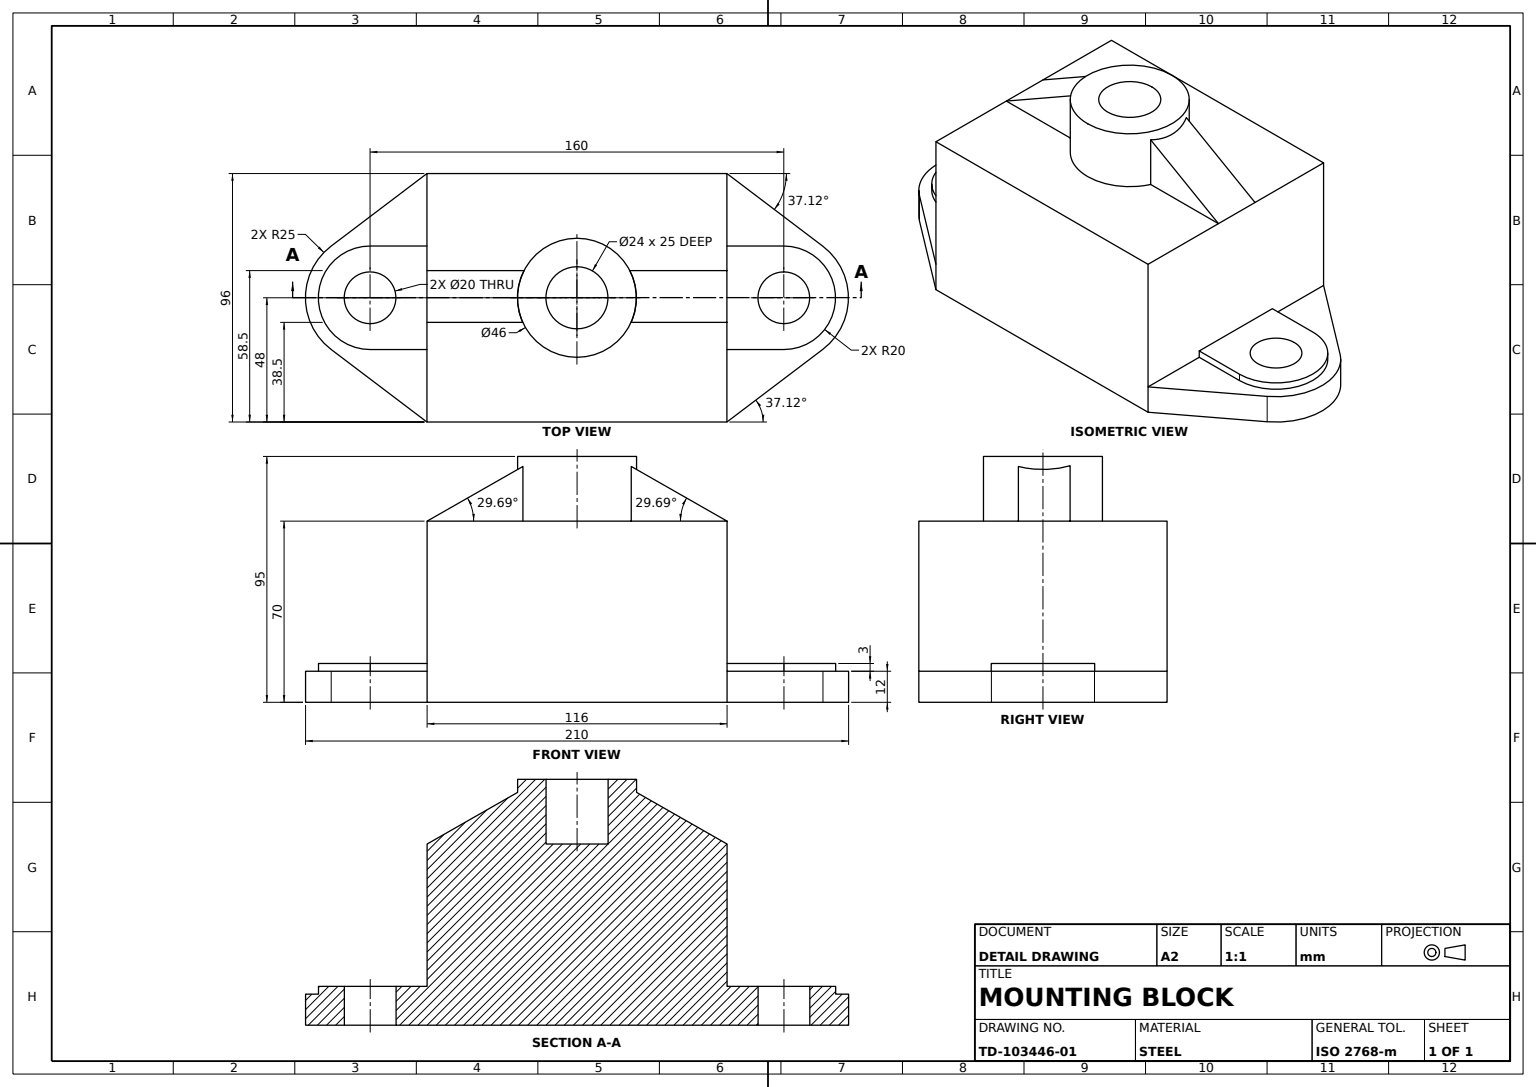
from build123d import *

# Parameters (mm, degrees)
HOUSING_BLOCK_SKETCH_W = 116
HOUSING_BLOCK_SKETCH_H = 70
HOUSING_BLOCK_DEPTH    = 96
MOUNTING_FLANGE_DEPTH  = 12
FLANGE_PAD_DEPTH       = 3
FLANGE_HOLE_SKETCH_R   = 10
FLANGE_HOLE_DEPTH      = 198.002538055
TOP_BOSS_SKETCH_R      = 23
TOP_BOSS_SKETCH_R_2    = 12
TOP_BOSS_46_DEPTH      = 25
GUSSET_DEPTH           = 10


with BuildPart() as part:
    # Housing Block Sketch → Housing Block (new body)
    with BuildSketch(Plane.XY):
        with Locations((58, 35)):
            Rectangle(HOUSING_BLOCK_SKETCH_W, HOUSING_BLOCK_SKETCH_H)
    extrude(amount=HOUSING_BLOCK_DEPTH)

    # Mounting Flange Sketch → Mounting Flange (add)
    with BuildSketch(Plane(origin=(0, 0, 0), x_dir=(1, 0, 0), z_dir=(0, 1, 0))):
        with BuildLine():
            Line((116, 0), (116, -96))
            Line((116, -96), (153.08596721, -67.935234971))
            ThreePointArc((153.08596721, -67.935234971), (163, -48), (153.08596721, -28.064765029))
            Line((153.08596721, -28.064765029), (116, 0))
        make_face()
    mounting_flange = extrude(amount=MOUNTING_FLANGE_DEPTH)

    # Flange Pad Sketch → Flange Pad (add)
    with BuildSketch(Plane(origin=(0, 12, 0), x_dir=(1, 0, 0), z_dir=(0, 1, 0))):
        with BuildLine():
            Line((138, -28), (116, -28))
            Line((116, -28), (116, -68))
            Line((116, -68), (138, -68))
            ThreePointArc((138, -68), (158, -48), (138, -28))
        make_face()
    flange_pad = extrude(amount=FLANGE_PAD_DEPTH)

    # Flange Hole Sketch → Flange Hole (cut, through all)
    with BuildSketch(Plane(origin=(0, 15, 0), x_dir=(1, 0, 0), z_dir=(0, 1, 0))):
        with Locations(Location((138, -48, 0), (0, 0, 270))):
            Circle(FLANGE_HOLE_SKETCH_R)
    flange_hole = extrude(amount=-FLANGE_HOLE_DEPTH, mode=Mode.SUBTRACT)

    # Flange Mirror: Mounting Flange, Flange Pad, Flange Hole across plane
    add(mounting_flange.mirror(Plane(origin=(58, 0, 0), x_dir=(0, 0, 1), z_dir=(1, 0, 0))))
    add(flange_pad.mirror(Plane(origin=(58, 0, 0), x_dir=(0, 0, 1), z_dir=(1, 0, 0))))
    add(flange_hole.mirror(Plane(origin=(58, 0, 0), x_dir=(0, 0, 1), z_dir=(1, 0, 0))), mode=Mode.SUBTRACT)

    # Top Boss Sketch → Top Boss Ø46 (add)
    with BuildSketch(Plane(origin=(0, 70, 0), x_dir=(1, 0, 0), z_dir=(0, 1, 0))):
        with Locations(Location((58, -48, 0), (0, 0, 90))):
            Circle(TOP_BOSS_SKETCH_R)
        with Locations(Location((58, -48, 0), (0, 0, 270))):
            Circle(TOP_BOSS_SKETCH_R_2, mode=Mode.SUBTRACT)
    extrude(amount=TOP_BOSS_46_DEPTH)

    # Gusset Sketch → Gusset (add, symmetric)
    with BuildSketch(Plane.XY.offset(47.5)):
        Polygon((81, 70), (116, 70), (72.155995343, 95), (72.155995343, 70), align=None)
    gusset = extrude(amount=GUSSET_DEPTH, both=True)

    # Gusset Mirror: Gusset across plane
    add(gusset.mirror(Plane(origin=(58, 0, 0), x_dir=(0, 0, 1), z_dir=(1, 0, 0))))


solid = part.part
